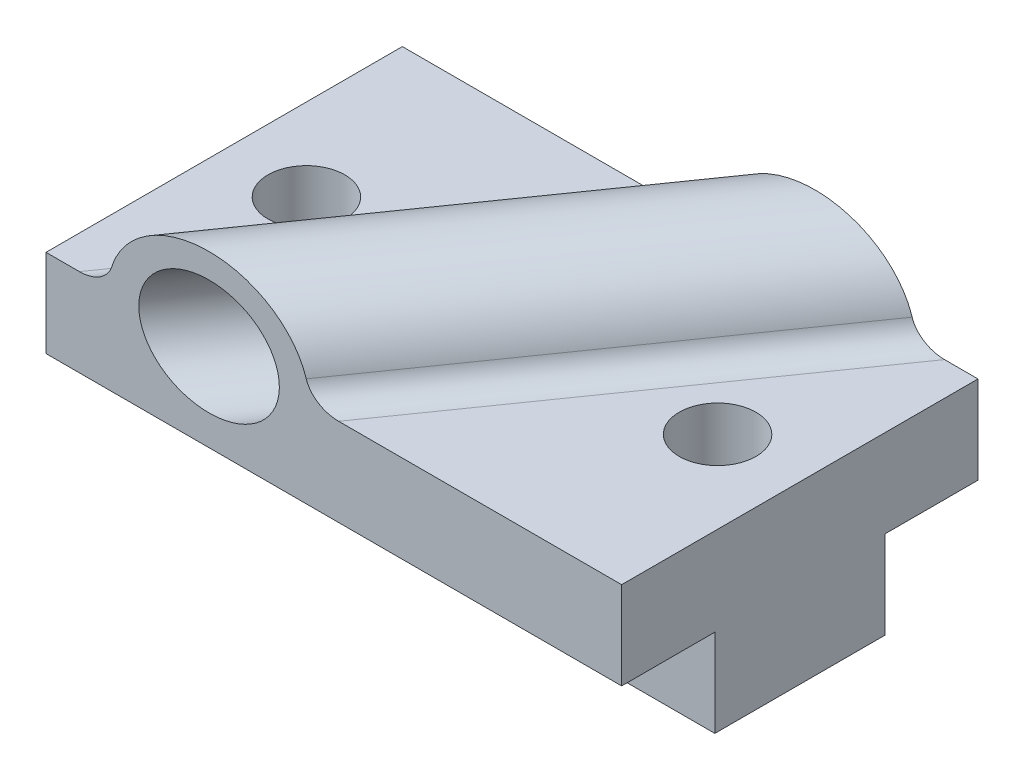
ISO-10303-21;
HEADER;
FILE_DESCRIPTION(('STEP AP214'),'2;1');
FILE_NAME('part.step','',(''),(''),'','','');
FILE_SCHEMA(('AUTOMOTIVE_DESIGN { 1 0 10303 214 1 1 1 1 }'));
ENDSEC;
DATA;
#1=APPLICATION_CONTEXT('core data for automotive mechanical design processes');
#2=APPLICATION_PROTOCOL_DEFINITION('international standard','automotive_design',2000,#1);
#3=PRODUCT_CONTEXT('',#1,'mechanical');
#4=PRODUCT('Part','Part','',(#3));
#5=PRODUCT_RELATED_PRODUCT_CATEGORY('part','',(#4));
#6=PRODUCT_DEFINITION_FORMATION('','',#4);
#7=PRODUCT_DEFINITION_CONTEXT('part definition',#1,'design');
#8=PRODUCT_DEFINITION('design','',#6,#7);
#9=PRODUCT_DEFINITION_SHAPE('','',#8);
#10=(LENGTH_UNIT() NAMED_UNIT(*) SI_UNIT(.MILLI.,.METRE.));
#11=(NAMED_UNIT(*) PLANE_ANGLE_UNIT() SI_UNIT($,.RADIAN.));
#12=(NAMED_UNIT(*) SI_UNIT($,.STERADIAN.) SOLID_ANGLE_UNIT());
#13=UNCERTAINTY_MEASURE_WITH_UNIT(LENGTH_MEASURE(1.E-05),#10,'distance_accuracy_value','');
#14=(GEOMETRIC_REPRESENTATION_CONTEXT(3) GLOBAL_UNCERTAINTY_ASSIGNED_CONTEXT((#13)) GLOBAL_UNIT_ASSIGNED_CONTEXT((#10,
#11,#12)) REPRESENTATION_CONTEXT('',''));
#15=CARTESIAN_POINT('',(0.,0.,0.));
#16=DIRECTION('',(0.,0.,1.));
#17=DIRECTION('',(1.,0.,0.));
#18=AXIS2_PLACEMENT_3D('',#15,#16,#17);
#19=CARTESIAN_POINT('',(0.,0.,0.));
#20=DIRECTION('',(0.,-1.,0.));
#21=DIRECTION('',(0.,0.,-1.));
#22=AXIS2_PLACEMENT_3D('',#19,#20,#21);
#23=PLANE('',#22);
#24=CARTESIAN_POINT('',(-37.5,1.20000000006226E-05,0.));
#25=DIRECTION('',(0.,1.,0.));
#26=DIRECTION('',(0.,0.,1.));
#27=AXIS2_PLACEMENT_3D('',#24,#25,#26);
#28=CIRCLE('',#27,7.);
#29=CARTESIAN_POINT('',(-37.5,1.20000000006226E-05,7.));
#30=VERTEX_POINT('',#29);
#31=EDGE_CURVE('E307',#30,#30,#28,.T.);
#32=ORIENTED_EDGE('',*,*,#31,.F.);
#33=EDGE_LOOP('',(#32));
#34=FACE_BOUND('',#33,.T.);
#35=DIRECTION('',(1.,0.,0.));
#36=VECTOR('',#35,1.);
#37=CARTESIAN_POINT('',(-52.5,0.,32.5));
#38=LINE('',#37,#36);
#39=CARTESIAN_POINT('',(-52.5,0.,32.5));
#40=VERTEX_POINT('',#39);
#41=CARTESIAN_POINT('',(-46.3969432505473,0.,32.5));
#42=VERTEX_POINT('',#41);
#43=EDGE_CURVE('E152',#40,#42,#38,.T.);
#44=ORIENTED_EDGE('',*,*,#43,.T.);
#45=DIRECTION('',(-0.573576436351047,0.,0.819152044288991));
#46=VECTOR('',#45,1.);
#47=CARTESIAN_POINT('',(0.869595697013503,0.,-35.0036133835573));
#48=LINE('',#47,#46);
#49=CARTESIAN_POINT('',(-0.883453266916023,0.,-32.5));
#50=VERTEX_POINT('',#49);
#51=EDGE_CURVE('E229',#42,#50,#48,.F.);
#52=ORIENTED_EDGE('',*,*,#51,.T.);
#53=DIRECTION('',(-1.,0.,0.));
#54=VECTOR('',#53,1.);
#55=CARTESIAN_POINT('',(-52.5,0.,-32.5));
#56=LINE('',#55,#54);
#57=CARTESIAN_POINT('',(-52.5,0.,-32.5));
#58=VERTEX_POINT('',#57);
#59=EDGE_CURVE('E172',#50,#58,#56,.T.);
#60=ORIENTED_EDGE('',*,*,#59,.T.);
#61=DIRECTION('',(0.,0.,1.));
#62=VECTOR('',#61,1.);
#63=CARTESIAN_POINT('',(-52.5,0.,32.5));
#64=LINE('',#63,#62);
#65=EDGE_CURVE('E180',#58,#40,#64,.T.);
#66=ORIENTED_EDGE('',*,*,#65,.T.);
#67=EDGE_LOOP('',(#44,#52,#60,#66));
#68=FACE_BOUND('',#67,.T.);
#69=ADVANCED_FACE('F39',(#34,#68),#23,.F.);
#70=CARTESIAN_POINT('',(37.5,1.20000000006226E-05,0.));
#71=DIRECTION('',(0.,1.,0.));
#72=DIRECTION('',(0.,0.,1.));
#73=AXIS2_PLACEMENT_3D('',#70,#71,#72);
#74=CIRCLE('',#73,7.);
#75=CARTESIAN_POINT('',(37.5,1.20000000006226E-05,7.));
#76=VERTEX_POINT('',#75);
#77=EDGE_CURVE('E191',#76,#76,#74,.T.);
#78=ORIENTED_EDGE('',*,*,#77,.F.);
#79=EDGE_LOOP('',(#78));
#80=FACE_BOUND('',#79,.T.);
#81=CARTESIAN_POINT('',(52.5,0.,-32.5));
#82=VERTEX_POINT('',#81);
#83=CARTESIAN_POINT('',(46.3969432505473,0.,-32.5));
#84=VERTEX_POINT('',#83);
#85=EDGE_CURVE('E174',#82,#84,#56,.T.);
#86=ORIENTED_EDGE('',*,*,#85,.T.);
#87=DIRECTION('',(-0.573576436351047,0.,0.819152044288991));
#88=VECTOR('',#87,1.);
#89=CARTESIAN_POINT('',(-0.869595697013531,0.,35.0036133835573));
#90=LINE('',#89,#88);
#91=CARTESIAN_POINT('',(0.88345326691603,0.,32.5));
#92=VERTEX_POINT('',#91);
#93=EDGE_CURVE('E58',#84,#92,#90,.T.);
#94=ORIENTED_EDGE('',*,*,#93,.T.);
#95=CARTESIAN_POINT('',(52.5,0.,32.5));
#96=VERTEX_POINT('',#95);
#97=EDGE_CURVE('E156',#92,#96,#38,.T.);
#98=ORIENTED_EDGE('',*,*,#97,.T.);
#99=DIRECTION('',(0.,0.,-1.));
#100=VECTOR('',#99,1.);
#101=CARTESIAN_POINT('',(52.5,0.,32.5));
#102=LINE('',#101,#100);
#103=EDGE_CURVE('E171',#96,#82,#102,.T.);
#104=ORIENTED_EDGE('',*,*,#103,.T.);
#105=EDGE_LOOP('',(#86,#94,#98,#104));
#106=FACE_BOUND('',#105,.T.);
#107=ADVANCED_FACE('F208',(#80,#106),#23,.F.);
#108=CARTESIAN_POINT('',(0.,-16.,0.));
#109=DIRECTION('',(0.,-1.,0.));
#110=DIRECTION('',(0.,0.,-1.));
#111=AXIS2_PLACEMENT_3D('',#108,#109,#110);
#112=PLANE('',#111);
#113=DIRECTION('',(0.,0.,-1.));
#114=VECTOR('',#113,1.);
#115=CARTESIAN_POINT('',(52.5,-16.,32.5));
#116=LINE('',#115,#114);
#117=CARTESIAN_POINT('',(52.5,-16.,-15.5));
#118=VERTEX_POINT('',#117);
#119=CARTESIAN_POINT('',(52.5,-16.,-32.5));
#120=VERTEX_POINT('',#119);
#121=EDGE_CURVE('E131',#118,#120,#116,.T.);
#122=ORIENTED_EDGE('',*,*,#121,.F.);
#123=DIRECTION('',(-1.,0.,0.));
#124=VECTOR('',#123,1.);
#125=CARTESIAN_POINT('',(87.3855270850248,-16.,-15.5));
#126=LINE('',#125,#124);
#127=CARTESIAN_POINT('',(-52.5,-16.,-15.5));
#128=VERTEX_POINT('',#127);
#129=EDGE_CURVE('E136',#118,#128,#126,.T.);
#130=ORIENTED_EDGE('',*,*,#129,.T.);
#131=DIRECTION('',(0.,0.,1.));
#132=VECTOR('',#131,1.);
#133=CARTESIAN_POINT('',(-52.5,-16.,32.5));
#134=LINE('',#133,#132);
#135=CARTESIAN_POINT('',(-52.5,-16.,-32.5));
#136=VERTEX_POINT('',#135);
#137=EDGE_CURVE('E164',#136,#128,#134,.T.);
#138=ORIENTED_EDGE('',*,*,#137,.F.);
#139=DIRECTION('',(-1.,0.,0.));
#140=VECTOR('',#139,1.);
#141=CARTESIAN_POINT('',(-52.5,-16.,-32.5));
#142=LINE('',#141,#140);
#143=EDGE_CURVE('E155',#120,#136,#142,.T.);
#144=ORIENTED_EDGE('',*,*,#143,.F.);
#145=EDGE_LOOP('',(#122,#130,#138,#144));
#146=FACE_BOUND('',#145,.T.);
#147=ADVANCED_FACE('F148',(#146),#112,.T.);
#148=CARTESIAN_POINT('',(52.5,-16.,32.5));
#149=DIRECTION('',(1.,0.,0.));
#150=DIRECTION('',(0.,0.,-1.));
#151=AXIS2_PLACEMENT_3D('',#148,#149,#150);
#152=PLANE('',#151);
#153=ORIENTED_EDGE('',*,*,#103,.F.);
#154=DIRECTION('',(0.,1.,0.));
#155=VECTOR('',#154,1.);
#156=CARTESIAN_POINT('',(52.5,-16.,32.5));
#157=LINE('',#156,#155);
#158=CARTESIAN_POINT('',(52.5,-16.,32.5));
#159=VERTEX_POINT('',#158);
#160=EDGE_CURVE('E179',#159,#96,#157,.T.);
#161=ORIENTED_EDGE('',*,*,#160,.F.);
#162=CARTESIAN_POINT('',(52.5,-16.,15.5));
#163=VERTEX_POINT('',#162);
#164=EDGE_CURVE('E153',#159,#163,#116,.T.);
#165=ORIENTED_EDGE('',*,*,#164,.T.);
#166=DIRECTION('',(0.,1.,0.));
#167=VECTOR('',#166,1.);
#168=CARTESIAN_POINT('',(52.5,-16.,15.5));
#169=LINE('',#168,#167);
#170=CARTESIAN_POINT('',(52.5,-32.,15.5));
#171=VERTEX_POINT('',#170);
#172=EDGE_CURVE('E268',#171,#163,#169,.T.);
#173=ORIENTED_EDGE('',*,*,#172,.F.);
#174=DIRECTION('',(0.,0.,1.));
#175=VECTOR('',#174,1.);
#176=CARTESIAN_POINT('',(52.5,-32.,-15.5));
#177=LINE('',#176,#175);
#178=CARTESIAN_POINT('',(52.5,-32.,-15.5));
#179=VERTEX_POINT('',#178);
#180=EDGE_CURVE('E132',#179,#171,#177,.T.);
#181=ORIENTED_EDGE('',*,*,#180,.F.);
#182=DIRECTION('',(0.,-1.,0.));
#183=VECTOR('',#182,1.);
#184=CARTESIAN_POINT('',(52.5,-16.,-15.5));
#185=LINE('',#184,#183);
#186=EDGE_CURVE('E127',#118,#179,#185,.T.);
#187=ORIENTED_EDGE('',*,*,#186,.F.);
#188=ORIENTED_EDGE('',*,*,#121,.T.);
#189=DIRECTION('',(0.,1.,0.));
#190=VECTOR('',#189,1.);
#191=CARTESIAN_POINT('',(52.5,-16.,-32.5));
#192=LINE('',#191,#190);
#193=EDGE_CURVE('E167',#120,#82,#192,.T.);
#194=ORIENTED_EDGE('',*,*,#193,.T.);
#195=EDGE_LOOP('',(#153,#161,#165,#173,#181,#187,#188,#194));
#196=FACE_BOUND('',#195,.T.);
#197=ADVANCED_FACE('F126',(#196),#152,.T.);
#198=CARTESIAN_POINT('',(-52.5,-16.,32.5));
#199=DIRECTION('',(0.,0.,1.));
#200=DIRECTION('',(1.,0.,0.));
#201=AXIS2_PLACEMENT_3D('',#198,#199,#200);
#202=PLANE('',#201);
#203=CARTESIAN_POINT('',(-22.7567449918156,0.,32.5));
#204=DIRECTION('',(0.,0.,1.));
#205=DIRECTION('',(1.,0.,0.));
#206=AXIS2_PLACEMENT_3D('',#203,#204,#205);
#207=ELLIPSE('',#206,12.8181331819953,10.5);
#208=CARTESIAN_POINT('',(-9.93861180982034,0.,32.5));
#209=VERTEX_POINT('',#208);
#210=EDGE_CURVE('E300',#209,#209,#207,.T.);
#211=ORIENTED_EDGE('',*,*,#210,.F.);
#212=EDGE_LOOP('',(#211));
#213=FACE_BOUND('',#212,.T.);
#214=ORIENTED_EDGE('',*,*,#97,.F.);
#215=CARTESIAN_POINT('',(0.883453266916023,5.,32.5));
#216=DIRECTION('',(0.,0.,1.));
#217=DIRECTION('',(1.,0.,0.));
#218=AXIS2_PLACEMENT_3D('',#215,#216,#217);
#219=ELLIPSE('',#218,6.10387294380729,5.);
#220=CARTESIAN_POINT('',(-5.02659629776689,3.75,32.5));
#221=VERTEX_POINT('',#220);
#222=EDGE_CURVE('E11',#92,#221,#219,.F.);
#223=ORIENTED_EDGE('',*,*,#222,.T.);
#224=CARTESIAN_POINT('',(-22.7567449918156,0.,32.5));
#225=DIRECTION('',(0.,0.,1.));
#226=DIRECTION('',(1.,0.,0.));
#227=AXIS2_PLACEMENT_3D('',#224,#225,#226);
#228=ELLIPSE('',#227,18.3116188314219,15.);
#229=CARTESIAN_POINT('',(-40.4868936858644,3.75,32.5));
#230=VERTEX_POINT('',#229);
#231=EDGE_CURVE('E253',#221,#230,#228,.T.);
#232=ORIENTED_EDGE('',*,*,#231,.T.);
#233=CARTESIAN_POINT('',(-46.3969432505473,5.,32.5));
#234=DIRECTION('',(0.,0.,1.));
#235=DIRECTION('',(1.,0.,0.));
#236=AXIS2_PLACEMENT_3D('',#233,#234,#235);
#237=ELLIPSE('',#236,6.10387294380729,5.);
#238=EDGE_CURVE('E231',#230,#42,#237,.F.);
#239=ORIENTED_EDGE('',*,*,#238,.T.);
#240=ORIENTED_EDGE('',*,*,#43,.F.);
#241=DIRECTION('',(0.,1.,0.));
#242=VECTOR('',#241,1.);
#243=CARTESIAN_POINT('',(-52.5,-16.,32.5));
#244=LINE('',#243,#242);
#245=CARTESIAN_POINT('',(-52.5,-16.,32.5));
#246=VERTEX_POINT('',#245);
#247=EDGE_CURVE('E183',#246,#40,#244,.T.);
#248=ORIENTED_EDGE('',*,*,#247,.F.);
#249=DIRECTION('',(1.,0.,0.));
#250=VECTOR('',#249,1.);
#251=CARTESIAN_POINT('',(-52.5,-16.,32.5));
#252=LINE('',#251,#250);
#253=EDGE_CURVE('E170',#246,#159,#252,.T.);
#254=ORIENTED_EDGE('',*,*,#253,.T.);
#255=ORIENTED_EDGE('',*,*,#160,.T.);
#256=EDGE_LOOP('',(#214,#223,#232,#239,#240,#248,#254,#255));
#257=FACE_BOUND('',#256,.T.);
#258=ADVANCED_FACE('F211',(#213,#257),#202,.T.);
#259=CARTESIAN_POINT('',(-52.5,-16.,32.5));
#260=DIRECTION('',(-1.,0.,0.));
#261=DIRECTION('',(0.,0.,1.));
#262=AXIS2_PLACEMENT_3D('',#259,#260,#261);
#263=PLANE('',#262);
#264=ORIENTED_EDGE('',*,*,#65,.F.);
#265=DIRECTION('',(0.,1.,0.));
#266=VECTOR('',#265,1.);
#267=CARTESIAN_POINT('',(-52.5,-16.,-32.5));
#268=LINE('',#267,#266);
#269=EDGE_CURVE('E187',#136,#58,#268,.T.);
#270=ORIENTED_EDGE('',*,*,#269,.F.);
#271=ORIENTED_EDGE('',*,*,#137,.T.);
#272=DIRECTION('',(0.,-1.,0.));
#273=VECTOR('',#272,1.);
#274=CARTESIAN_POINT('',(-52.5,-16.,-15.5));
#275=LINE('',#274,#273);
#276=CARTESIAN_POINT('',(-52.5,-32.,-15.5));
#277=VERTEX_POINT('',#276);
#278=EDGE_CURVE('E141',#128,#277,#275,.T.);
#279=ORIENTED_EDGE('',*,*,#278,.T.);
#280=DIRECTION('',(0.,0.,1.));
#281=VECTOR('',#280,1.);
#282=CARTESIAN_POINT('',(-52.5,-32.,-15.5));
#283=LINE('',#282,#281);
#284=CARTESIAN_POINT('',(-52.5,-32.,15.5));
#285=VERTEX_POINT('',#284);
#286=EDGE_CURVE('E150',#277,#285,#283,.T.);
#287=ORIENTED_EDGE('',*,*,#286,.T.);
#288=DIRECTION('',(0.,1.,0.));
#289=VECTOR('',#288,1.);
#290=CARTESIAN_POINT('',(-52.5,-16.,15.5));
#291=LINE('',#290,#289);
#292=CARTESIAN_POINT('',(-52.5,-16.,15.5));
#293=VERTEX_POINT('',#292);
#294=EDGE_CURVE('E308',#285,#293,#291,.T.);
#295=ORIENTED_EDGE('',*,*,#294,.T.);
#296=EDGE_CURVE('E165',#293,#246,#134,.T.);
#297=ORIENTED_EDGE('',*,*,#296,.T.);
#298=ORIENTED_EDGE('',*,*,#247,.T.);
#299=EDGE_LOOP('',(#264,#270,#271,#279,#287,#295,#297,#298));
#300=FACE_BOUND('',#299,.T.);
#301=ADVANCED_FACE('F256',(#300),#263,.T.);
#302=CARTESIAN_POINT('',(-52.5,-16.,-32.5));
#303=DIRECTION('',(0.,0.,-1.));
#304=DIRECTION('',(-1.,0.,0.));
#305=AXIS2_PLACEMENT_3D('',#302,#303,#304);
#306=PLANE('',#305);
#307=CARTESIAN_POINT('',(22.7567449918156,0.,-32.5));
#308=DIRECTION('',(0.,0.,-1.));
#309=DIRECTION('',(-1.,0.,0.));
#310=AXIS2_PLACEMENT_3D('',#307,#308,#309);
#311=ELLIPSE('',#310,12.8181331819953,10.5);
#312=CARTESIAN_POINT('',(9.93861180982034,0.,-32.5));
#313=VERTEX_POINT('',#312);
#314=EDGE_CURVE('E248',#313,#313,#311,.F.);
#315=ORIENTED_EDGE('',*,*,#314,.T.);
#316=EDGE_LOOP('',(#315));
#317=FACE_BOUND('',#316,.T.);
#318=ORIENTED_EDGE('',*,*,#59,.F.);
#319=CARTESIAN_POINT('',(-0.883453266916037,5.,-32.5));
#320=DIRECTION('',(0.,0.,-1.));
#321=DIRECTION('',(1.,0.,0.));
#322=AXIS2_PLACEMENT_3D('',#319,#320,#321);
#323=ELLIPSE('',#322,6.10387294380729,5.);
#324=CARTESIAN_POINT('',(5.02659629776689,3.75,-32.5));
#325=VERTEX_POINT('',#324);
#326=EDGE_CURVE('E232',#50,#325,#323,.F.);
#327=ORIENTED_EDGE('',*,*,#326,.T.);
#328=CARTESIAN_POINT('',(22.7567449918156,0.,-32.5));
#329=DIRECTION('',(0.,0.,-1.));
#330=DIRECTION('',(-1.,0.,0.));
#331=AXIS2_PLACEMENT_3D('',#328,#329,#330);
#332=ELLIPSE('',#331,18.3116188314219,15.);
#333=CARTESIAN_POINT('',(40.4868936858644,3.75,-32.5));
#334=VERTEX_POINT('',#333);
#335=EDGE_CURVE('E239',#334,#325,#332,.F.);
#336=ORIENTED_EDGE('',*,*,#335,.F.);
#337=CARTESIAN_POINT('',(46.3969432505473,5.,-32.5));
#338=DIRECTION('',(0.,0.,-1.));
#339=DIRECTION('',(1.,0.,0.));
#340=AXIS2_PLACEMENT_3D('',#337,#338,#339);
#341=ELLIPSE('',#340,6.10387294380729,5.);
#342=EDGE_CURVE('E50',#334,#84,#341,.F.);
#343=ORIENTED_EDGE('',*,*,#342,.T.);
#344=ORIENTED_EDGE('',*,*,#85,.F.);
#345=ORIENTED_EDGE('',*,*,#193,.F.);
#346=ORIENTED_EDGE('',*,*,#143,.T.);
#347=ORIENTED_EDGE('',*,*,#269,.T.);
#348=EDGE_LOOP('',(#318,#327,#336,#343,#344,#345,#346,#347));
#349=FACE_BOUND('',#348,.T.);
#350=ADVANCED_FACE('F237',(#317,#349),#306,.T.);
#351=DIRECTION('',(-1.,0.,0.));
#352=VECTOR('',#351,1.);
#353=CARTESIAN_POINT('',(87.3855270850248,-16.,15.5));
#354=LINE('',#353,#352);
#355=EDGE_CURVE('E162',#163,#293,#354,.T.);
#356=ORIENTED_EDGE('',*,*,#355,.F.);
#357=ORIENTED_EDGE('',*,*,#164,.F.);
#358=ORIENTED_EDGE('',*,*,#253,.F.);
#359=ORIENTED_EDGE('',*,*,#296,.F.);
#360=EDGE_LOOP('',(#356,#357,#358,#359));
#361=FACE_BOUND('',#360,.T.);
#362=ADVANCED_FACE('F215',(#361),#112,.T.);
#363=CARTESIAN_POINT('',(87.3855270850248,-16.,-15.5));
#364=DIRECTION('',(0.,0.,-1.));
#365=DIRECTION('',(0.,1.,0.));
#366=AXIS2_PLACEMENT_3D('',#363,#364,#365);
#367=PLANE('',#366);
#368=ORIENTED_EDGE('',*,*,#129,.F.);
#369=ORIENTED_EDGE('',*,*,#186,.T.);
#370=DIRECTION('',(-1.,0.,0.));
#371=VECTOR('',#370,1.);
#372=CARTESIAN_POINT('',(87.3855270850248,-32.,-15.5));
#373=LINE('',#372,#371);
#374=EDGE_CURVE('E140',#179,#277,#373,.T.);
#375=ORIENTED_EDGE('',*,*,#374,.T.);
#376=ORIENTED_EDGE('',*,*,#278,.F.);
#377=EDGE_LOOP('',(#368,#369,#375,#376));
#378=FACE_BOUND('',#377,.T.);
#379=ADVANCED_FACE('F142',(#378),#367,.T.);
#380=CARTESIAN_POINT('',(87.3855270850248,-32.,-15.5));
#381=DIRECTION('',(0.,-1.,0.));
#382=DIRECTION('',(0.,0.,-1.));
#383=AXIS2_PLACEMENT_3D('',#380,#381,#382);
#384=PLANE('',#383);
#385=CARTESIAN_POINT('',(-37.5,-32.,0.));
#386=DIRECTION('',(0.,1.,0.));
#387=DIRECTION('',(0.,0.,1.));
#388=AXIS2_PLACEMENT_3D('',#385,#386,#387);
#389=CIRCLE('',#388,7.);
#390=CARTESIAN_POINT('',(-37.5,-32.,7.));
#391=VERTEX_POINT('',#390);
#392=EDGE_CURVE('E304',#391,#391,#389,.T.);
#393=ORIENTED_EDGE('',*,*,#392,.T.);
#394=EDGE_LOOP('',(#393));
#395=FACE_BOUND('',#394,.T.);
#396=CARTESIAN_POINT('',(37.5,-32.,0.));
#397=DIRECTION('',(0.,1.,0.));
#398=DIRECTION('',(0.,0.,1.));
#399=AXIS2_PLACEMENT_3D('',#396,#397,#398);
#400=CIRCLE('',#399,7.);
#401=CARTESIAN_POINT('',(37.5,-32.,7.));
#402=VERTEX_POINT('',#401);
#403=EDGE_CURVE('E297',#402,#402,#400,.T.);
#404=ORIENTED_EDGE('',*,*,#403,.T.);
#405=EDGE_LOOP('',(#404));
#406=FACE_BOUND('',#405,.T.);
#407=ORIENTED_EDGE('',*,*,#374,.F.);
#408=ORIENTED_EDGE('',*,*,#180,.T.);
#409=DIRECTION('',(-1.,0.,0.));
#410=VECTOR('',#409,1.);
#411=CARTESIAN_POINT('',(87.3855270850248,-32.,15.5));
#412=LINE('',#411,#410);
#413=EDGE_CURVE('E353',#171,#285,#412,.T.);
#414=ORIENTED_EDGE('',*,*,#413,.T.);
#415=ORIENTED_EDGE('',*,*,#286,.F.);
#416=EDGE_LOOP('',(#407,#408,#414,#415));
#417=FACE_BOUND('',#416,.T.);
#418=ADVANCED_FACE('F358',(#395,#406,#417),#384,.T.);
#419=CARTESIAN_POINT('',(87.3855270850248,-16.,15.5));
#420=DIRECTION('',(0.,0.,1.));
#421=DIRECTION('',(1.,0.,0.));
#422=AXIS2_PLACEMENT_3D('',#419,#420,#421);
#423=PLANE('',#422);
#424=ORIENTED_EDGE('',*,*,#413,.F.);
#425=ORIENTED_EDGE('',*,*,#172,.T.);
#426=ORIENTED_EDGE('',*,*,#355,.T.);
#427=ORIENTED_EDGE('',*,*,#294,.F.);
#428=EDGE_LOOP('',(#424,#425,#426,#427));
#429=FACE_BOUND('',#428,.T.);
#430=ADVANCED_FACE('F332',(#429),#423,.T.);
#431=CARTESIAN_POINT('',(37.5,-32.,0.));
#432=DIRECTION('',(0.,1.,0.));
#433=DIRECTION('',(0.,0.,1.));
#434=AXIS2_PLACEMENT_3D('',#431,#432,#433);
#435=CYLINDRICAL_SURFACE('',#434,7.);
#436=ORIENTED_EDGE('',*,*,#403,.F.);
#437=EDGE_LOOP('',(#436));
#438=FACE_BOUND('',#437,.T.);
#439=ORIENTED_EDGE('',*,*,#77,.T.);
#440=EDGE_LOOP('',(#439));
#441=FACE_BOUND('',#440,.T.);
#442=ADVANCED_FACE('F329',(#438,#441),#435,.F.);
#443=CARTESIAN_POINT('',(-37.5,-32.,0.));
#444=DIRECTION('',(0.,1.,0.));
#445=DIRECTION('',(0.,0.,1.));
#446=AXIS2_PLACEMENT_3D('',#443,#444,#445);
#447=CYLINDRICAL_SURFACE('',#446,7.);
#448=ORIENTED_EDGE('',*,*,#392,.F.);
#449=EDGE_LOOP('',(#448));
#450=FACE_BOUND('',#449,.T.);
#451=ORIENTED_EDGE('',*,*,#31,.T.);
#452=EDGE_LOOP('',(#451));
#453=FACE_BOUND('',#452,.T.);
#454=ADVANCED_FACE('F318',(#450,#453),#447,.F.);
#455=CARTESIAN_POINT('',(-49.7777835771756,0.,71.0900423957835));
#456=DIRECTION('',(0.573576436351047,0.,-0.819152044288991));
#457=DIRECTION('',(-0.819152044288991,0.,-0.573576436351047));
#458=AXIS2_PLACEMENT_3D('',#455,#456,#457);
#459=CYLINDRICAL_SURFACE('',#458,15.);
#460=ORIENTED_EDGE('',*,*,#335,.T.);
#461=DIRECTION('',(0.573576436351047,0.,-0.819152044288991));
#462=VECTOR('',#461,1.);
#463=CARTESIAN_POINT('',(-61.6748919229619,3.75,62.7595974491662));
#464=LINE('',#463,#462);
#465=EDGE_CURVE('E227',#325,#230,#464,.F.);
#466=ORIENTED_EDGE('',*,*,#465,.T.);
#467=ORIENTED_EDGE('',*,*,#231,.F.);
#468=DIRECTION('',(0.573576436351047,0.,-0.819152044288991));
#469=VECTOR('',#468,1.);
#470=CARTESIAN_POINT('',(-37.8806752313893,3.75,79.4204873424007));
#471=LINE('',#470,#469);
#472=EDGE_CURVE('E182',#221,#334,#471,.T.);
#473=ORIENTED_EDGE('',*,*,#472,.T.);
#474=EDGE_LOOP('',(#460,#466,#467,#473));
#475=FACE_BOUND('',#474,.T.);
#476=ADVANCED_FACE('F244',(#475),#459,.T.);
#477=CARTESIAN_POINT('',(-49.7777835771756,0.,71.0900423957835));
#478=DIRECTION('',(0.573576436351047,0.,-0.819152044288991));
#479=DIRECTION('',(-0.819152044288991,0.,-0.573576436351047));
#480=AXIS2_PLACEMENT_3D('',#477,#478,#479);
#481=CYLINDRICAL_SURFACE('',#480,10.5);
#482=ORIENTED_EDGE('',*,*,#314,.F.);
#483=EDGE_LOOP('',(#482));
#484=FACE_BOUND('',#483,.T.);
#485=ORIENTED_EDGE('',*,*,#210,.T.);
#486=EDGE_LOOP('',(#485));
#487=FACE_BOUND('',#486,.T.);
#488=ADVANCED_FACE('F274',(#484,#487),#481,.F.);
#489=CARTESIAN_POINT('',(-65.6405947048907,5.,59.9827824669605));
#490=DIRECTION('',(0.573576436351047,0.,-0.819152044288991));
#491=DIRECTION('',(-0.819152044288991,0.,-0.573576436351047));
#492=AXIS2_PLACEMENT_3D('',#489,#490,#491);
#493=CYLINDRICAL_SURFACE('',#492,5.);
#494=ORIENTED_EDGE('',*,*,#326,.F.);
#495=ORIENTED_EDGE('',*,*,#51,.F.);
#496=ORIENTED_EDGE('',*,*,#238,.F.);
#497=ORIENTED_EDGE('',*,*,#465,.F.);
#498=EDGE_LOOP('',(#494,#495,#496,#497));
#499=FACE_BOUND('',#498,.T.);
#500=ADVANCED_FACE('F252',(#499),#493,.F.);
#501=CARTESIAN_POINT('',(-33.9149724494605,5.,82.1973023246065));
#502=DIRECTION('',(0.573576436351047,0.,-0.819152044288991));
#503=DIRECTION('',(-0.819152044288991,0.,-0.573576436351047));
#504=AXIS2_PLACEMENT_3D('',#501,#502,#503);
#505=CYLINDRICAL_SURFACE('',#504,5.);
#506=ORIENTED_EDGE('',*,*,#222,.F.);
#507=ORIENTED_EDGE('',*,*,#93,.F.);
#508=ORIENTED_EDGE('',*,*,#342,.F.);
#509=ORIENTED_EDGE('',*,*,#472,.F.);
#510=EDGE_LOOP('',(#506,#507,#508,#509));
#511=FACE_BOUND('',#510,.T.);
#512=ADVANCED_FACE('F41',(#511),#505,.F.);
#513=CLOSED_SHELL('',(#69,#107,#147,#197,#258,#301,#350,#362,#379,#418,#430,#442,#454,#476,#488,
#500,#512));
#514=MANIFOLD_SOLID_BREP('B2',#513);
#515=ADVANCED_BREP_SHAPE_REPRESENTATION('',(#18,#514),#14);
#516=SHAPE_DEFINITION_REPRESENTATION(#9,#515);
ENDSEC;
END-ISO-10303-21;
